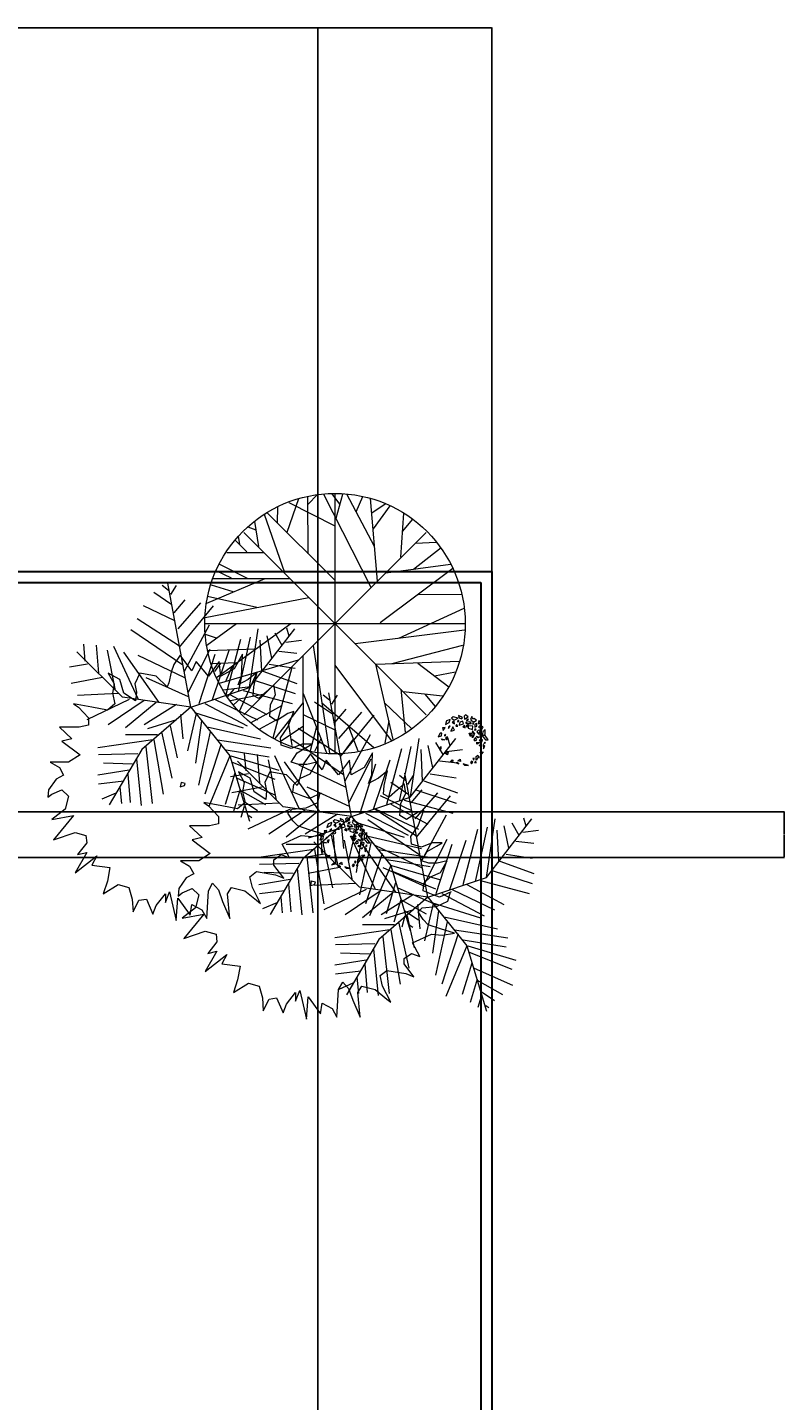
# Model space of a CAD drawing. Units: inches. Extents: x 2330 to 3943, y 1763 to 3461.
# Tile 40 of 40: x 3594 to 3943, y 2829 to 3461. Entities that reach past the tile are written whole.
import ezdxf

# ---------------------------------------------------------------- set-up
doc = ezdxf.new("R2010")
doc.units = ezdxf.units.IN
for name, color, linetype, lineweight in [('A-ANNO-DIMS', 2, 'Continuous', 18), ('C-PROP', 7, 'Continuous', 30), ('L-PLNT', 94, 'Continuous', 13)]:
    doc.layers.add(name, color=color, linetype=linetype, lineweight=lineweight)
doc.styles.get("Standard").update_dxf_attribs({"font": 'arial.ttf'})
doc.dimstyles.get("Standard").update_dxf_attribs({"dimtxt": 0.18, "dimasz": 0.18, "dimexe": 0.18, "dimexo": 0.0625, "dimgap": 0.09, "dimtad": 0, "dimtih": 1, "dimtoh": 1, "dimdec": 4, "dimzin": 0, "dimdsep": 46, "dimtxsty": 'Standard', "dimcen": 0.09, "dimadec": 0, "dimazin": 0, "dimtfac": 1, "dimtdec": 4, "dimtofl": 0, "dimtmove": 0, "dimatfit": 3, "dimfxl": 1, "dimtolj": 1, "dimtzin": 0, "dimarcsym": 0})

# ---------------------------------------------------------------- blocks, each defined once
blk = doc.blocks.new('*U12')
for p, q in [((0, 0), (-10.5, 57)), ((-8.737, 47.138), (-17.069, 52.711)), ((-10.186, 53.64), (-13.084, 55.962)), ((-9.099, 51.782), (-6.563, 55.962)), ((-7.288, 39.707), (-21.778, 46.673)), ((-7.65, 43.423), (-2.578, 49.46)), ((-5.839, 35.992), (4.667, 48.067)), ((-5.114, 27.632), (10.463, 46.673)), ((-5.114, 28.097), (-24.676, 40.636)), ((-3.665, 19.273), (-27.574, 35.527)), ((-2.941, 16.486), (8.652, 37.85)), ((22.055, 7.198), (27.489, 32.277)), ((27, 9), (48, 36)), ((27.127, 9.056), (31.112, 35.992)), ((35.096, 32.741), (37.27, 22.524)), ((38.719, 34.134), (41.979, 28.561)), ((44.153, 36.456), (45.239, 32.741)), ((-31.5, 4.5), (-52.5, 25.5)), ((-48.585, 21.131), (-49.309, 29.026)), ((-43.513, 28.561), (-42.427, 15.558)), ((-38.442, 26.239), (-34.819, 7.663)), ((-35.544, 28.097), (-24.314, 3.947)), ((-14.533, 2.09), (-30.834, 25.31)), ((-1.129, 6.734), (9.014, 26.704)), ((10.101, 3.483), (17.708, 26.239)), ((16.259, 5.805), (23.142, 31.348)), ((31.836, 30.883), (32.561, 16.486)), ((40.53, 25.775), (48.862, 24.846)), ((43.791, 29.954), (51.036, 30.883)), ((-47.498, 19.737), (-55.83, 18.344)), ((-24.314, 23.917), (-2.941, 13.7)), ((3.942, 1.625), (11.187, 24.381)), ((36.183, 19.737), (48.137, 17.88)), ((-40.615, 13.7), (-55.105, 10.913)), ((-20.691, 13.7), (-1.129, 4.876)), ((33.285, 16.486), (48.862, 10.913)), ((0, 0), (27, 9)), ((24.229, 7.663), (46.688, 1.625)), ((29.662, 12.307), (48.137, 6.269)), ((-33.37, 6.269), (-52.207, 5.34)), ((-28.299, 3.483), (-47.86, -5.805)), ((-21.416, 3.018), (-38.079, -8.128)), ((0, 0), (-31.5, 4.5)), ((-15.982, 2.09), (-30.11, -9.521)), ((0, 0), (-22.5, -19.5)), ((-6.563, 1.161), (-21.416, -8.128)), ((0, 0), (18, -22.5)), ((6.478, 1.625), (26.04, -8.592)), ((11.187, 3.483), (30.749, -5.805)), ((18.07, 5.805), (35.096, -3.483)), ((-6.563, -5.805), (-19.967, -9.985)), ((-4.752, -3.483), (-3.665, -14.629)), ((2.493, -3.019), (-1.491, -20.202)), ((1.769, -2.555), (24.229, -9.521)), ((5.029, -6.27), (2.131, -25.775)), ((-13.446, -11.378), (-8.737, -32.741)), ((-9.461, -8.592), (-6.201, -23.453)), ((9.014, -11.378), (3.58, -35.992)), ((7.565, -9.056), (32.198, -14.629)), ((-17.431, -15.094), (-42.789, -18.809)), ((-15.257, -12.772), (-30.11, -12.772)), ((-20.691, -18.345), (-17.793, -44.352)), ((-17.069, -15.094), (-12.721, -40.172)), ((14.085, -16.951), (6.478, -40.172)), ((12.274, -15.094), (36.907, -18.809)), ((-24.314, -21.596), (-42.427, -22.06)), ((-22.5, -19.5), (-37.5, -45)), ((-25.038, -23.918), (-22.865, -45.281)), ((18.07, -22.524), (8.289, -45.745)), ((16.259, -19.738), (36.183, -22.989)), ((18, -22.5), (27, -52.5)), ((18.433, -22.524), (40.53, -29.026)), ((-28.299, -29.026), (-42.789, -31.348)), ((-26.849, -26.24), (-40.253, -25.775)), ((-29.023, -30.884), (-27.936, -43.887)), ((20.244, -30.419), (15.897, -44.816)), ((19.157, -25.311), (38.719, -33.206)), ((-30.834, -34.135), (-42.427, -35.528)), ((-32.646, -36.921), (-31.921, -44.352)), ((22.78, -37.85), (19.519, -48.532)), ((21.331, -32.741), (39.081, -40.636)), ((-34.457, -39.708), (-40.978, -42.494)), ((22.78, -38.314), (34.372, -44.816)), ((24.591, -43.423), (30.749, -47.603)), ((24.591, -45.745), (23.142, -50.854)), ((26.764, -49.925), (28.213, -50.854))]:
    blk.add_line(p, q)
blk = doc.blocks.new('*U14')
for p, q in [((-22.0458, 42.0753), (-16.5881, 57.6486)), ((-12.5388, 54.9406), (-7.9613, 59.4546)), ((-12.3627, 32.1443), (-12.5388, 58.7776)), ((-5.3205, 59.6806), (16.5105, 16.7963)), ((2.426, 54.9406), (-1.4472, 59.9056)), ((0, 59.9996), (0, -60)), ((0.4894, 48.6208), (3.6584, 59.6806)), ((18.2711, 35.5298), (5.419, 59.6806)), ((9.8203, 51.5549), (12.8133, 58.5516)), ((19.6795, 19.5047), (16.3344, 57.6486)), ((-31.2008, 51.1035), (-0.2149, 20.1818)), ((-26.4472, 46.5894), (-26.2712, 53.8116)), ((-21.1656, 55.8436), (-0.0388, 45.0094)), ((17.0387, 51.1035), (23.2006, 55.1666)), ((17.7429, 43.6552), (25.4894, 54.2636)), ((31.6513, 50.8778), (30.2429, 30.5643)), ((-40.1797, 44.558), (-36.4825, 43.2038)), ((-37.0107, 47.0408), (-35.25, 35.5298)), ((-32.6092, 50.4264), (-23.2782, 23.5674)), ((31.1232, 42.5267), (35.8767, 48.1693)), ((-45.8134, 38.2383), (-40.5318, 33.0471)), ((-43.8768, 36.4326), (-44.405, 40.2696)), ((42, 42), (-42, -42)), ((42, -42), (-42, 42)), ((-49.8627, 32.8214), (-32.7853, 32.8214)), ((36.2288, 25.1474), (48.9049, 35.0784)), ((37.1091, 37.1098), (46.6161, 37.5612)), ((-53.2078, 27.4044), (-40.1797, 20.859)), ((54.3626, 25.3731), (20.9119, 0.3198)), ((23.3767, 23.3417), (53.3063, 27.4044)), ((-32.2571, 20.6333), (-59.1937, 9.348)), ((-56.0247, 20.859), (-20.8134, 20.859)), ((-54.7923, 24.4702), (-47.75, 21.0847)), ((-58.6656, 12.7336), (-35.9543, 7.5424)), ((-57.081, 17.9248), (-47.0458, 14.7649)), ((38.5175, 13.4107), (58.2359, 13.6364)), ((-59.7219, 2.8025), (-12.0106, 12.0565)), ((29.3626, -6.6771), (59.4682, 7.091)), ((-54.6162, -24.7335), (-20.2853, 0.0941)), ((-60, 0), (60, 0)), ((-59.7219, -4.8714), (-54.2641, -6.6771)), ((-45.2853, -0.1316), (-59.0177, -10.0627)), ((9.2922, -9.1598), (59.6443, -2.8401)), ((-58.4895, -12.3197), (-36.4825, -11.6426)), ((-10.074, -10.0627), (-2.5036, -59.7178)), ((26.3697, -18.4138), (58.9401, -9.8369)), ((-57.081, -18.4138), (-45.2853, -17.9624)), ((-52.6797, -18.188), (-55.4966, -22.0251)), ((-53.2078, -27.442), (-16.7641, -16.6081)), ((-14.8275, -15.0282), (-14.6515, -57.6865)), ((18.6232, -18.6394), (26.7218, -53.3981)), ((18.7992, -18.6394), (57.3556, -17.2853)), ((38.1654, -18.188), (52.426, -29.0219)), ((-47.2219, -19.3166), (-50.2148, -26.3135)), ((-35.9543, -22.4765), (-44.0529, -40.5329)), ((-19.9331, -20.2194), (-28.5599, -52.721)), ((-0.0388, -19.0909), (25.8415, -53.8495)), ((45.9119, -24.0564), (55.595, -22.2508)), ((-38.9472, -29.0219), (-51.4472, -30.6018)), ((-46.5177, -30.1504), (-49.5106, -33.536)), ((30.419, -30.1504), (32.3556, -50.0125)), ((31.4753, -31.279), (49.6091, -33.3103)), ((-32.4331, -32.4075), (-48.1021, -35.5674)), ((-43.7008, -34.6645), (-46.6937, -37.373)), ((-24.6867, -37.8244), (-38.7712, -45.7241)), ((-14.6515, -36.2445), (-27.6797, -52.9467)), ((-14.6515, -32.1818), (-3.912, -59.4922)), ((-6.2008, -36.2445), (17.919, -57.0094)), ((22.8485, -36.4702), (35.3485, -48.4326)), ((41.5105, -32.6332), (46.088, -38.0501)), ((-26.2712, -43.9185), (-34.7219, -48.6583)), ((-14.6515, -47.3041), (-25.0388, -54.3009)), ((-21.5177, -45.4984), (-19.9331, -56.1065)), ((-8.4895, -47.5298), (-11.4825, -58.5893)), ((5.9471, -46.6269), (10.5246, -58.5893)), ((24.7852, -44.8213), (23.0246, -54.978)), ((-6.3768, -52.721), (-9.3698, -58.815)), ((8.4119, -53.1724), (3.8344, -59.4922))]:
    blk.add_line(p, q)
blk.add_circle((0, 0), 60)
blk = doc.blocks.new('*U15')
for points in [[(0, 60.64), (-3.051, 56.238), (-4.196, 52.815), (-5.34, 47.925), (-6.103, 45.969), (-11.062, 50.859), (-18.691, 52.326), (-20.98, 47.436), (-20.217, 43.524), (-20.598, 39.611), (-25.939, 43.035), (-27.846, 49.392), (-33.186, 52.326), (-30.516, 47.436), (-31.279, 43.035), (-30.135, 38.144), (-33.568, 35.21), (-40.815, 36.677), (-49.208, 38.144), (-46.919, 36.677), (-42.341, 31.787), (-42.341, 28.364), (-46.537, 27.386), (-55.692, 27.386), (-49.97, 22.006), (-54.548, 21.028), (-46.156, 14.671), (-51.496, 11.248), (-59.888, 11.248), (-55.692, 8.803), (-53.785, 5.38), (-57.218, 3.423), (-60.651, -1.467), (-61.033, -4.89), (-59.125, -3.423), (-54.548, -1.467), (-51.496, -4.401), (-53.022, -10.269), (-59.125, -15.16), (-49.208, -13.204), (-58.362, -24.451), (-48.445, -21.028), (-43.486, -22.495), (-43.104, -25.918), (-47.3, -31.298), (-43.104, -30.32), (-48.445, -39.611), (-38.527, -31.787), (-40.815, -36.188), (-32.423, -37.166), (-33.568, -43.523), (-35.475, -49.392), (-28.609, -44.99), (-23.65, -46.457), (-22.124, -51.837), (-21.743, -57.705), (-19.073, -52.326), (-15.639, -51.837), (-12.588, -58.683), (-11.062, -54.771), (-6.866, -49.392), (-6.866, -53.304), (-4.959, -48.414), (-1.907, -61.617), (-1.144, -51.348), (4.578, -59.172), (5.341, -54.282), (9.918, -56.727), (12.207, -60.639), (12.97, -47.925), (14.877, -44.501), (17.547, -47.436), (19.455, -52.815), (22.888, -60.639), (21.743, -49.392), (23.65, -46.457), (29.754, -47.925), (35.094, -52.326), (37.001, -53.793), (33.187, -46.457), (32.042, -41.567), (35.094, -39.122), (43.868, -40.589), (47.682, -42.056), (43.105, -36.188), (43.105, -33.743), (46.538, -31.298), (50.352, -32.765), (46.919, -26.407), (55.693, -22.495), (60.652, -22.984), (66.374, -22.006), (59.889, -20.05), (54.167, -18.094), (51.878, -15.649), (49.589, -12.225), (51.497, -10.269), (57.981, -9.78), (63.322, -7.335), (64.466, -2.934)], [(64.848, -2.934), (59.507, -5.379), (56.456, -4.401), (51.878, -2.445), (52.26, 0.978), (55.311, 3.912), (59.889, 5.869), (62.94, 11.248), (58.363, 10.27), (54.548, 10.27), (51.115, 11.248), (53.785, 15.649), (57.981, 18.094), (60.652, 19.561), (56.074, 19.561), (51.115, 17.605), (46.538, 19.072), (46.156, 22.496), (49.589, 27.386), (52.26, 34.721), (49.589, 33.743), (44.249, 30.32), (41.197, 32.276), (41.579, 37.655), (43.868, 42.546), (43.105, 46.947), (40.053, 44.013), (36.238, 40.589), (33.568, 42.057), (33.95, 45.969), (35.476, 52.815), (31.28, 49.392), (26.702, 46.947), (28.228, 50.859), (28.609, 61.129), (24.795, 54.282), (18.692, 50.859), (17.929, 57.706), (12.97, 50.859), (7.248, 57.706), (5.341, 53.304), (0, 60.64)]]:
    blk.add_lwpolyline(points)
blk.add_lwpolyline([(0.382, 1.956), (0, 0), (1.907, 0.489), (2.289, 1.467)], close=True)
blk = doc.blocks.new('*U13')
for points in [[(-5.78, 9.75), (-7.54, 9.23), (-8.01, 7.5), (-6.26, 8.45)], [(-5.78, 6.81), (-6.66, 6.21), (-6.52, 5.69)], [(-4.57, 6.38), (-5.45, 4.47), (-3.89, 4.82)], [(-4.43, 11.05), (-5.18, 10.36), (-3.96, 9.49), (-2.07, 10.36)], [(-4.84, 8.63), (-3.83, 7.85), (-4.03, 8.97)], [(-2.88, 7.5), (-3.15, 6.64), (-2.27, 6.72)], [(-1.94, 9.49), (-2.48, 8.97), (-2.27, 8.54), (-1.8, 9.06)], [(-2, 11.66), (-1.6, 10.62), (-0.52, 10.1), (-0.18, 10.62), (-0.79, 10.96)], [(0.02, 9.06), (-1.33, 8.54), (-1.73, 7.16), (0.29, 7.76)], [(0.76, 7.16), (0.09, 6.46), (1.1, 5.95)], [(1.24, 12), (0.56, 11.31), (0.76, 10.01), (2.52, 11.05)], [(1.37, 8.54), (3.13, 8.8), (3.8, 7.85), (1.91, 7.76)], [(2.59, 9.93), (1.84, 9.75), (1.64, 9.23), (2.32, 9.41)], [(1.71, 6.29), (1.71, 7.07), (2.65, 7.5), (2.11, 6.9)], [(2.52, 6.81), (2.52, 5.86), (4.41, 5.17), (4.61, 6.72)], [(4.14, 11.14), (3.6, 10.01), (4, 9.23), (5.22, 8.71), (6.3, 9.41), (5.08, 10.19), (4.61, 10.01)], [(4.61, 8.28), (4.54, 7.76), (4.95, 7.59), (4.95, 8.28)], [(6.43, 7.94), (5.49, 7.68), (5.56, 6.21), (6.5, 6.64)], [(7.45, 9.32), (7.11, 7.94), (8.52, 7.94)], [(7.85, 6.81), (7.18, 6.21), (9, 5.51), (9.33, 6.38)], [(-11.32, 1.79), (-9.83, 2.31), (-9.63, 3.44), (-10.44, 3.52)], [(-8.21, 0.41), (-9.43, 0.32), (-9.83, 0.84)], [(-8.14, 6.03), (-9.36, 5.95), (-9.02, 4.73)], [(-8.21, 3.09), (-8.48, 2.31), (-7.87, 2.57)], [(-7, 1.79), (-7.94, 1.53), (-7.47, 0.49)], [(3.53, 1.88), (2.86, 3.52), (3.8, 3.52)], [(4.41, 4.56), (4.27, 3.7), (5.49, 3.26)], [(4.27, 2.74), (5.29, 2.66), (4.41, 1.27)], [(5.83, 1.53), (5.02, 0.41), (5.49, -0.02), (6.5, 0.41)], [(5.49, 5.51), (5.42, 4.82), (6.16, 5.08)], [(7.51, 1.71), (6.91, 1.27), (6.23, 2.14)], [(8.12, 4.99), (7.11, 4.65), (6.5, 4.13), (7.38, 3.09), (8.12, 3.52), (7.65, 3.87)], [(8.12, 0.75), (7.51, 0.15), (8.93, -0.28), (9.13, 0.49)], [(8.19, 2.57), (7.92, 2.05), (8.66, 1.53)], [(8.73, 4.73), (8.19, 4.56), (8.39, 3.87), (8.59, 4.04)], [(10.28, 5.17), (9.2, 4.04), (9, 2.31), (10.48, 0.49), (11.76, 0.41), (10.35, 2.48), (9.33, 2.4), (10.28, 2.83)], [(-10.03, -2.71), (-10.64, -3.31), (-10.44, -4.44), (-9.9, -3.49)], [(-8.28, -5.73), (-6.79, -5.3), (-7, -6.51)], [(7.78, -0.8), (6.43, -1.5), (6.43, -0.72)], [(8.32, -1.75), (7.98, -2.53), (7.58, -2.1)], [(9.33, -5.13), (8.46, -6.25), (7.98, -5.22)], [(9.33, -1.75), (9.54, -3.74), (10.14, -2.53)], [(10.08, -0.63), (9.74, -1.32), (10.48, -0.89)], [(-4.84, -8.85), (-4.43, -9.45), (-5.99, -9.8)], [(-2.54, -10.06), (-3.02, -10.23), (-1.8, -10.67)], [(-2.34, -9.2), (-1.26, -8.5), (-0.99, -9.54)], [(0.22, -10.58), (0.83, -11.27), (2.59, -11.36)], [(4.07, -9.45), (3.53, -9.97), (4.07, -10.58), (4.61, -9.89)], [(5.29, -7.98), (4.61, -8.16), (5.02, -8.94)], [(6.03, -9.45), (5.42, -9.97), (6.16, -10.15)], [(6.1, -8.94), (6.16, -7.21), (6.91, -6.69), (7.24, -7.38)], [(8.05, -8.07), (8.59, -7.12), (7.92, -7.55)]]:
    blk.add_lwpolyline(points, close=True)
blk = doc.blocks.new('*D59')
at = {"layer": 'A-ANNO-DIMS', "color": 0, "lineweight": -2, "transparency": 16777216}
for p, q in [((2415.66, 3210.71), (2415.66, 3461.3)), ((2415.84, 3461.12), (3111.31, 3461.12)), ((3807.48, 3461.12), (3112.01, 3461.12)), ((3807.66, 3210.71), (3807.66, 3461.3))]:
    blk.add_line(p, q, dxfattribs=at)
at = {"layer": 'A-ANNO-DIMS', "color": 0, "transparency": 16777216}
for points in [[(2415.84, 3461.15), (2415.84, 3461.09), (2415.66, 3461.12)], [(3807.48, 3461.15), (3807.48, 3461.09), (3807.66, 3461.12)]]:
    blk.add_solid(points, dxfattribs=at)
at = {"layer": 'Defpoints', "color": 0, "transparency": 16777216}
for p in [(3807.66, 3461.12), (2415.66, 3210.65), (3807.66, 3210.65)]:
    blk.add_point(p, dxfattribs=at)
at = {"layer": 'A-ANNO-DIMS', "color": 0, "transparency": 16777216, "insert": (3111.66, 3461.12), "char_height": 0.18, "attachment_point": 5}
blk.add_mtext('\\A1;1392', dxfattribs=at)
blk = doc.blocks.new('*D67')
at = {"layer": 'A-ANNO-DIMS', "color": 0, "lineweight": -2, "transparency": 16777216}
for p, q in [((3727.52, 2560.76), (3727.52, 3461.3)), ((3727.7, 3461.12), (3767.19, 3461.12)), ((3807.48, 3461.12), (3767.98, 3461.12)), ((3807.66, 2560.76), (3807.66, 3461.3))]:
    blk.add_line(p, q, dxfattribs=at)
at = {"layer": 'A-ANNO-DIMS', "color": 0, "transparency": 16777216}
for points in [[(3727.7, 3461.15), (3727.7, 3461.09), (3727.52, 3461.12)], [(3807.48, 3461.15), (3807.48, 3461.09), (3807.66, 3461.12)]]:
    blk.add_solid(points, dxfattribs=at)
at = {"layer": 'Defpoints', "color": 0, "transparency": 16777216}
for p in [(3807.66, 3461.12), (3727.52, 2560.7), (3807.66, 2560.7)]:
    blk.add_point(p, dxfattribs=at)
at = {"layer": 'A-ANNO-DIMS', "color": 0, "transparency": 16777216, "insert": (3767.59, 3461.12), "char_height": 0.18, "attachment_point": 5}
blk.add_mtext('\\A1;80.14', dxfattribs=at)
blk = doc.blocks.new('*D86')
at = {"layer": 'A-ANNO-DIMS', "color": 0, "lineweight": -2, "transparency": 16777216}
for p, q in [((2979.18, 3100.04), (3942.54, 3100.04)), ((3942.36, 3099.86), (3942.36, 3089.72)), ((3942.36, 3079.22), (3942.36, 3089.36)), ((2979.18, 3079.04), (3942.54, 3079.04))]:
    blk.add_line(p, q, dxfattribs=at)
at = {"layer": 'A-ANNO-DIMS', "color": 0, "transparency": 16777216}
for points in [[(3942.33, 3099.86), (3942.39, 3099.86), (3942.36, 3100.04)], [(3942.33, 3079.22), (3942.39, 3079.22), (3942.36, 3079.04)]]:
    blk.add_solid(points, dxfattribs=at)
at = {"layer": 'Defpoints', "color": 0, "transparency": 16777216}
for p in [(2979.12, 3100.04), (2979.12, 3079.04), (3942.36, 3079.04)]:
    blk.add_point(p, dxfattribs=at)
at = {"layer": 'A-ANNO-DIMS', "color": 0, "transparency": 16777216, "insert": (3942.36, 3089.54), "char_height": 0.18, "attachment_point": 5}
blk.add_mtext('\\A1;21', dxfattribs=at)

msp = doc.modelspace()

# ---------------------------------------------------------------- linework, layer by layer
at = {"layer": 'C-PROP'}
for p, q in [((2415.6605, 3210.6524), (3807.6605, 3210.6524)), ((3807.6605, 3210.6524), (3807.6605, 1974.6524)), ((2420.6605, 3205.6524), (3802.6605, 3205.6524)), ((3802.6605, 3205.6524), (3802.6605, 2560.7019))]:
    msp.add_line(p, q, dxfattribs=at)

# ---------------------------------------------------------------- block references
at = {"layer": 'L-PLNT'}
for name, p in [('*U14', (3735.4199, 3186.6811)), ('*U12', (3668.9889, 3148.2594)), ('*U15', (3664.1819, 3111.5784)), ('*U12', (3743.0941, 3097.7891)), ('*U13', (3794.32, 3132.7509)), ('*U15', (3724.1567, 3066.1176)), ('*U12', (3778.1717, 3060.7416)), ('*U13', (3739.772, 3085.3149))]:
    msp.add_blockref(name, p, dxfattribs=at)

# ---------------------------------------------------------------- dimensions: what is measured, and where the dimension line sits
at = {"layer": 'A-ANNO-DIMS'}
for p1, p2, override, picture, middle in [((2415.6605, 3210.6524), (3807.6605, 3210.6524), {"dimdec": 0, "dimlfac": 1, "dimrnd": 0, "dimzin": 0, "dimdsep": 46, "dimlunit": 2}, '*D59', (3111.6605, 3461.1231)), ((3727.5159, 2560.7019), (3807.6605, 2560.7019), {"dimdec": 2, "dimlfac": 1, "dimrnd": 0, "dimzin": 0, "dimdsep": 46, "dimlunit": 2}, '*D67', (3767.5882, 3461.1231))]:
    dim = msp.add_linear_dim(base=(3807.6605, 3461.1231), p1=p1, p2=p2, dimstyle='Standard', override=override, dxfattribs=at)
    dim.commit()
    dim.dimension.update_dxf_attribs({"geometry": picture, "text_midpoint": middle})
dim = msp.add_linear_dim(base=(3942.361, 3079.0386), p1=(2979.1218, 3100.0386), p2=(2979.1218, 3079.0386), angle=90, dimstyle='Standard', override={"dimdec": 0, "dimlfac": 1, "dimrnd": 0, "dimzin": 0, "dimdsep": 46, "dimlunit": 2}, dxfattribs=at)
dim.commit()
dim.dimension.update_dxf_attribs({"geometry": '*D86', "text_midpoint": (3942.361, 3089.5386)})

doc.saveas('drawing.dxf')
